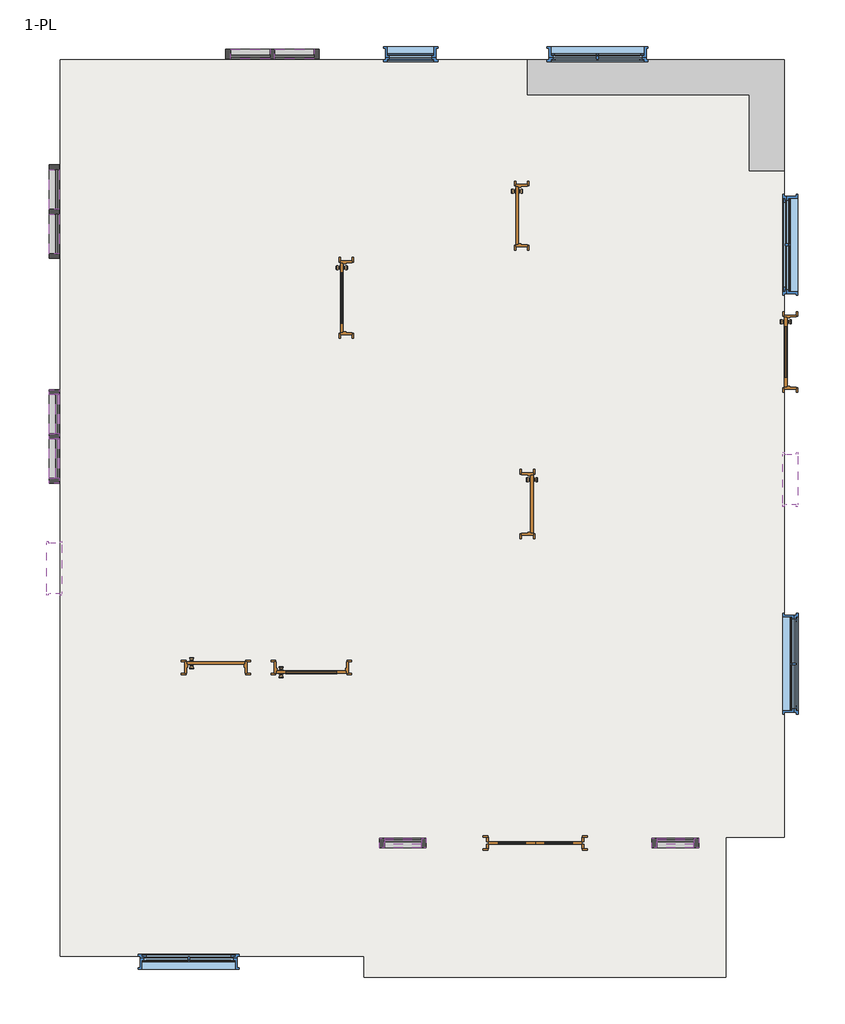
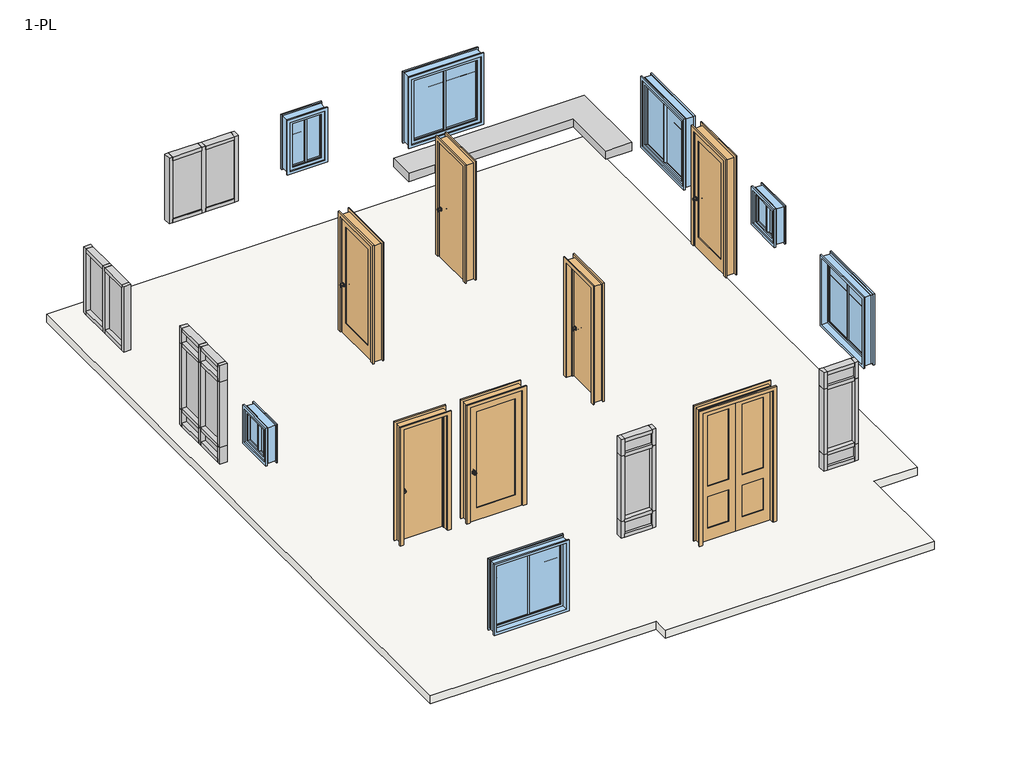
# One storey: 51 members, 16 plates, 7 doors, 7 windows, 1 furniture element, 1 slab.
"""IFC4 building model written with IfcOpenShell, lengths in millimetres."""

from ifc_helpers import new_model, si_unit, frame, origin, place, context, project, spatial, polyline, outline, extrude, transform, mapped, element, save
from components import door_interior_double_pocket_2_panel_wood_4_x8_0aea24c3, door_interior_single_1_panel_wood_3_x7_5a860750, door_2b62d641, door_6764305a, casework_1_casework_1_03657681, member_86d06fe4, member_323df77c, member_3c3dc66a, member_75074519, member_0b7646a3, member_75d1e245, member_aaa03826, member_2b49869a, system_panel_glazed_cd2dd794, system_panel_glazed_63160b6e, system_panel_glazed_17912afe, system_panel_glazed_1715a493, system_panel_solid_a8a40995, yu_window_casement_1219x1219_b0d26e5b, yu_window_casement_610x610_b7484dfd, yu_window_casement_610x914_cab7b646

model = new_model("IFC4")

# Units and contexts
model_context = context("Model", 3, world=origin())
ifc_project = project(units=[si_unit("LENGTHUNIT", "METRE", prefix="MILLI")], contexts=[model_context])

# Site, building, storey
site = spatial("IfcSite", under=ifc_project)
building = spatial("IfcBuilding", under=site)
storey = spatial("IfcBuildingStorey", under=building, Name="1-PL", Elevation=609.6)

# Doors
placement = place(None, origin())
door_interior_double_pocket_2_panel_wood_4_x8_shape = door_interior_double_pocket_2_panel_wood_4_x8_0aea24c3(model_context)
element("IfcDoor", 1, ObjectType="Door-Interior-Double-Pocket-2_Panel-Wood : 4'x8'", at=placement, inside=storey, context=model_context, shape_type="MappedRepresentation", body=[
    mapped(door_interior_double_pocket_2_panel_wood_4_x8_shape, transform((456.1465688, 1034.5352197, 609.6), x_axis=(-1.0, 0.0, 0.0), y_axis=(0.0, -1.0, 0.0), z_axis=(0.0, 0.0, 1.0))),
])
door_interior_single_1_panel_wood_3_x7_shape = door_interior_single_1_panel_wood_3_x7_5a860750(model_context)
element("IfcDoor", 2, ObjectType="Door-Interior-Single-1_Panel-Wood : 3'x7'", at=placement, inside=storey, context=model_context, shape_type="MappedRepresentation", body=[
    mapped(door_interior_single_1_panel_wood_3_x7_shape, transform((-2464.8534312, 3317.3602197, 609.6), x_axis=(1.0, 0.0, 0.0), y_axis=(0.0, 1.0, 0.0), z_axis=(0.0, 0.0, 1.0))),
])
element("IfcDoor", 3, ObjectType="Door-Interior-Single-1_Panel-Wood : 3'x7'", at=placement, inside=storey, context=model_context, shape_type="MappedRepresentation", body=[
    mapped(door_interior_single_1_panel_wood_3_x7_shape, transform((-2010.8284312, 8140.986397, 609.6), x_axis=(0.0, -1.0, 0.0), y_axis=(1.0, 0.0, 0.0), z_axis=(0.0, 0.0, 1.0))),
])
element("IfcDoor", 4, ObjectType="Door-Interior-Single-1_Panel-Wood : 3'x7'", at=placement, inside=storey, context=model_context, shape_type="MappedRepresentation", body=[
    mapped(door_interior_single_1_panel_wood_3_x7_shape, transform((3780.3715688, 7435.3352197, 609.6), x_axis=(0.0, -1.0, 0.0), y_axis=(1.0, 0.0, 0.0), z_axis=(0.0, 0.0, 1.0))),
])
door_shape = door_2b62d641(model_context)
element("IfcDoor", 5, ObjectType="Door-Interior-Single-Flush_Panel-Wood : 2'6\" x 7'", at=placement, inside=storey, context=model_context, shape_type="MappedRepresentation", body=[
    mapped(door_shape, transform((-3709.4534312, 3323.7102197, 609.6), x_axis=(1.0, 0.0, 0.0), y_axis=(0.0, 1.0, 0.0), z_axis=(0.0, 0.0, 1.0))),
])
element("IfcDoor", 6, ObjectType="Door-Interior-Single-Flush_Panel-Wood : 2'6\" x 7'", at=placement, inside=storey, context=model_context, shape_type="MappedRepresentation", body=[
    mapped(door_shape, transform((357.7215688, 5454.1352197, 609.6), x_axis=(0.0, -1.0, 0.0), y_axis=(1.0, 0.0, 0.0), z_axis=(0.0, 0.0, 1.0))),
])
door_2_shape = door_6764305a(model_context)
element("IfcDoor", 7, ObjectType="Door-Interior-Single-Flush_Panel-Wood : 2'6\" x 7'", at=placement, inside=storey, context=model_context, shape_type="MappedRepresentation", body=[
    mapped(door_2_shape, transform((275.1715688, 9213.3352197, 609.6), x_axis=(0.0, -1.0, 0.0), y_axis=(1.0, 0.0, 0.0), z_axis=(0.0, 0.0, 1.0))),
])

# Furniture
casework_1_casework_1_shape = casework_1_casework_1_03657681(model_context)
element("IfcFurniture", 8, ObjectType="Casework 1 : Casework 1", at=placement, inside=storey, context=model_context, shape_type="MappedRepresentation", body=[
    mapped(casework_1_casework_1_shape, transform((0.0, 0.0, 0.0), x_axis=(1.0, 0.0, 0.0), y_axis=(0.0, 1.0, 0.0), z_axis=(0.0, 0.0, 1.0))),
])

# Members
member_shape = member_86d06fe4(model_context)
element("IfcMember", 9, ObjectType="Rectangular Mullion : 2.5\" x 5\" rectangular", at=placement, inside=storey, context=model_context, shape_type="MappedRepresentation", body=[
    mapped(member_shape, transform((-1029.7534312, 1034.5352197, 3048.0), x_axis=(0.0, 0.0, 1.0), y_axis=(0.0, -1.0, 0.0), z_axis=(1.0, 0.0, 0.0))),
])
element("IfcMember", 10, ObjectType="Rectangular Mullion : 2.5\" x 5\" rectangular", at=placement, inside=storey, context=model_context, shape_type="MappedRepresentation", body=[
    mapped(member_shape, transform((2526.2465688, 1034.5352197, 3048.0), x_axis=(0.0, 0.0, 1.0), y_axis=(0.0, -1.0, 0.0), z_axis=(1.0, 0.0, 0.0))),
])
element("IfcMember", 11, ObjectType="Rectangular Mullion : 2.5\" x 5\" rectangular", at=placement, inside=storey, context=model_context, shape_type="MappedRepresentation", body=[
    mapped(member_shape, transform((-1512.3534312, 1034.5352197, 1219.2), x_axis=(0.0, 0.0, -1.0), y_axis=(0.0, -1.0, 0.0), z_axis=(-1.0, 0.0, 0.0))),
])
element("IfcMember", 12, ObjectType="Rectangular Mullion : 2.5\" x 5\" rectangular", at=placement, inside=storey, context=model_context, shape_type="MappedRepresentation", body=[
    mapped(member_shape, transform((2043.6465688, 1034.5352197, 1219.2), x_axis=(0.0, 0.0, -1.0), y_axis=(0.0, -1.0, 0.0), z_axis=(-1.0, 0.0, 0.0))),
])
member_2_shape = member_323df77c(model_context)
element("IfcMember", 13, ObjectType="Rectangular Mullion : 2.5\" x 5\" rectangular", at=placement, inside=storey, context=model_context, shape_type="MappedRepresentation", body=[
    mapped(member_2_shape, transform((-1029.7534312, 1034.5352197, 2743.2), x_axis=(0.0, 0.0, 1.0), y_axis=(0.0, -1.0, 0.0), z_axis=(1.0, 0.0, 0.0))),
])
element("IfcMember", 14, ObjectType="Rectangular Mullion : 2.5\" x 5\" rectangular", at=placement, inside=storey, context=model_context, shape_type="MappedRepresentation", body=[
    mapped(member_2_shape, transform((-1029.7534312, 1034.5352197, 1524.0), x_axis=(0.0, 0.0, 1.0), y_axis=(0.0, -1.0, 0.0), z_axis=(1.0, 0.0, 0.0))),
])
element("IfcMember", 15, ObjectType="Rectangular Mullion : 2.5\" x 5\" rectangular", at=placement, inside=storey, context=model_context, shape_type="MappedRepresentation", body=[
    mapped(member_2_shape, transform((2526.2465688, 1034.5352197, 2743.2), x_axis=(0.0, 0.0, 1.0), y_axis=(0.0, -1.0, 0.0), z_axis=(1.0, 0.0, 0.0))),
])
element("IfcMember", 16, ObjectType="Rectangular Mullion : 2.5\" x 5\" rectangular", at=placement, inside=storey, context=model_context, shape_type="MappedRepresentation", body=[
    mapped(member_2_shape, transform((2526.2465688, 1034.5352197, 1524.0), x_axis=(0.0, 0.0, 1.0), y_axis=(0.0, -1.0, 0.0), z_axis=(1.0, 0.0, 0.0))),
])
member_3_shape = member_3c3dc66a(model_context)
element("IfcMember", 17, ObjectType="Rectangular Mullion : 2.5\" x 5\" rectangular", at=placement, inside=storey, context=model_context, shape_type="MappedRepresentation", body=[
    mapped(member_3_shape, transform((-1575.8534312, 1034.5352197, 3048.0), x_axis=(-1.0, 0.0, 0.0), y_axis=(0.0, -1.0, 0.0), z_axis=(0.0, 0.0, 1.0))),
])
element("IfcMember", 18, ObjectType="Rectangular Mullion : 2.5\" x 5\" rectangular", at=placement, inside=storey, context=model_context, shape_type="MappedRepresentation", body=[
    mapped(member_3_shape, transform((1980.1465688, 1034.5352197, 3048.0), x_axis=(-1.0, 0.0, 0.0), y_axis=(0.0, -1.0, 0.0), z_axis=(0.0, 0.0, 1.0))),
])
element("IfcMember", 19, ObjectType="Rectangular Mullion : 2.5\" x 5\" rectangular", at=placement, inside=storey, context=model_context, shape_type="MappedRepresentation", body=[
    mapped(member_3_shape, transform((-5817.6534312, 6946.3852197, 3048.0), x_axis=(0.0, 1.0, 0.0), y_axis=(-1.0, 0.0, 0.0), z_axis=(0.0, 0.0, 1.0))),
])
element("IfcMember", 20, ObjectType="Rectangular Mullion : 2.5\" x 5\" rectangular", at=placement, inside=storey, context=model_context, shape_type="MappedRepresentation", body=[
    mapped(member_3_shape, transform((-966.2534312, 1034.5352197, 1219.2), x_axis=(1.0, 0.0, 0.0), y_axis=(0.0, -1.0, 0.0), z_axis=(0.0, 0.0, -1.0))),
])
element("IfcMember", 21, ObjectType="Rectangular Mullion : 2.5\" x 5\" rectangular", at=placement, inside=storey, context=model_context, shape_type="MappedRepresentation", body=[
    mapped(member_3_shape, transform((2589.7465688, 1034.5352197, 1219.2), x_axis=(1.0, 0.0, 0.0), y_axis=(0.0, -1.0, 0.0), z_axis=(0.0, 0.0, -1.0))),
])
element("IfcMember", 22, ObjectType="Rectangular Mullion : 2.5\" x 5\" rectangular", at=placement, inside=storey, context=model_context, shape_type="MappedRepresentation", body=[
    mapped(member_3_shape, transform((-5817.6534312, 5727.1852197, 1219.2), x_axis=(0.0, -1.0, 0.0), y_axis=(-1.0, 0.0, 0.0), z_axis=(0.0, 0.0, -1.0))),
])
element("IfcMember", 23, ObjectType="Rectangular Mullion : 2.5\" x 5\" rectangular", at=placement, inside=storey, context=model_context, shape_type="MappedRepresentation", body=[
    mapped(member_3_shape, transform((-966.2534312, 1034.5352197, 2743.2), x_axis=(1.0, 0.0, 0.0), y_axis=(0.0, -1.0, 0.0), z_axis=(0.0, 0.0, -1.0))),
])
element("IfcMember", 24, ObjectType="Rectangular Mullion : 2.5\" x 5\" rectangular", at=placement, inside=storey, context=model_context, shape_type="MappedRepresentation", body=[
    mapped(member_3_shape, transform((2589.7465688, 1034.5352197, 2743.2), x_axis=(1.0, 0.0, 0.0), y_axis=(0.0, -1.0, 0.0), z_axis=(0.0, 0.0, -1.0))),
])
element("IfcMember", 25, ObjectType="Rectangular Mullion : 2.5\" x 5\" rectangular", at=placement, inside=storey, context=model_context, shape_type="MappedRepresentation", body=[
    mapped(member_3_shape, transform((-5817.6534312, 5727.1852197, 2743.2), x_axis=(0.0, -1.0, 0.0), y_axis=(-1.0, 0.0, 0.0), z_axis=(0.0, 0.0, -1.0))),
])
member_4_shape = member_75074519(model_context)
element("IfcMember", 26, ObjectType="Rectangular Mullion : 2.5\" x 5\" rectangular", at=placement, inside=storey, context=model_context, shape_type="MappedRepresentation", body=[
    mapped(member_4_shape, transform((-966.2534312, 1034.5352197, 1524.0), x_axis=(1.0, 0.0, 0.0), y_axis=(0.0, -1.0, 0.0), z_axis=(0.0, 0.0, -1.0))),
])
element("IfcMember", 27, ObjectType="Rectangular Mullion : 2.5\" x 5\" rectangular", at=placement, inside=storey, context=model_context, shape_type="MappedRepresentation", body=[
    mapped(member_4_shape, transform((2589.7465688, 1034.5352197, 1524.0), x_axis=(1.0, 0.0, 0.0), y_axis=(0.0, -1.0, 0.0), z_axis=(0.0, 0.0, -1.0))),
])
element("IfcMember", 28, ObjectType="Rectangular Mullion : 2.5\" x 5\" rectangular", at=placement, inside=storey, context=model_context, shape_type="MappedRepresentation", body=[
    mapped(member_4_shape, transform((-5817.6534312, 5727.1852197, 1524.0), x_axis=(0.0, -1.0, 0.0), y_axis=(-1.0, 0.0, 0.0), z_axis=(0.0, 0.0, -1.0))),
])
element("IfcMember", 29, ObjectType="Rectangular Mullion : 2.5\" x 5\" rectangular", at=placement, inside=storey, context=model_context, shape_type="MappedRepresentation", body=[
    mapped(member_4_shape, transform((-1575.8534312, 1034.5352197, 2743.2), x_axis=(-1.0, 0.0, 0.0), y_axis=(0.0, -1.0, 0.0), z_axis=(0.0, 0.0, 1.0))),
])
element("IfcMember", 30, ObjectType="Rectangular Mullion : 2.5\" x 5\" rectangular", at=placement, inside=storey, context=model_context, shape_type="MappedRepresentation", body=[
    mapped(member_4_shape, transform((1980.1465688, 1034.5352197, 2743.2), x_axis=(-1.0, 0.0, 0.0), y_axis=(0.0, -1.0, 0.0), z_axis=(0.0, 0.0, 1.0))),
])
element("IfcMember", 31, ObjectType="Rectangular Mullion : 2.5\" x 5\" rectangular", at=placement, inside=storey, context=model_context, shape_type="MappedRepresentation", body=[
    mapped(member_4_shape, transform((-5817.6534312, 6946.3852197, 2743.2), x_axis=(0.0, 1.0, 0.0), y_axis=(-1.0, 0.0, 0.0), z_axis=(0.0, 0.0, 1.0))),
])
element("IfcMember", 32, ObjectType="Rectangular Mullion : 2.5\" x 5\" rectangular", at=placement, inside=storey, context=model_context, shape_type="MappedRepresentation", body=[
    mapped(member_3_shape, transform((-1575.8534312, 1034.5352197, 1524.0), x_axis=(-1.0, 0.0, 0.0), y_axis=(0.0, -1.0, 0.0), z_axis=(0.0, 0.0, 1.0))),
])
element("IfcMember", 33, ObjectType="Rectangular Mullion : 2.5\" x 5\" rectangular", at=placement, inside=storey, context=model_context, shape_type="MappedRepresentation", body=[
    mapped(member_3_shape, transform((1980.1465688, 1034.5352197, 1524.0), x_axis=(-1.0, 0.0, 0.0), y_axis=(0.0, -1.0, 0.0), z_axis=(0.0, 0.0, 1.0))),
])
element("IfcMember", 34, ObjectType="Rectangular Mullion : 2.5\" x 5\" rectangular", at=placement, inside=storey, context=model_context, shape_type="MappedRepresentation", body=[
    mapped(member_3_shape, transform((-5817.6534312, 6946.3852197, 1524.0), x_axis=(0.0, 1.0, 0.0), y_axis=(-1.0, 0.0, 0.0), z_axis=(0.0, 0.0, 1.0))),
])
member_5_shape = member_0b7646a3(model_context)
element("IfcMember", 35, ObjectType="Rectangular Mullion : 2.5\" x 5\" rectangular", at=placement, inside=storey, context=model_context, shape_type="MappedRepresentation", body=[
    mapped(member_5_shape, transform((-5817.6534312, 5790.6852197, 3048.0), x_axis=(0.0, 0.0, 1.0), y_axis=(-1.0, 0.0, 0.0), z_axis=(0.0, -1.0, 0.0))),
])
element("IfcMember", 36, ObjectType="Rectangular Mullion : 2.5\" x 5\" rectangular", at=placement, inside=storey, context=model_context, shape_type="MappedRepresentation", body=[
    mapped(member_5_shape, transform((-5817.6534312, 6368.5352197, 3048.0), x_axis=(0.0, 0.0, 1.0), y_axis=(-1.0, 0.0, 0.0), z_axis=(0.0, -1.0, 0.0))),
])
element("IfcMember", 37, ObjectType="Rectangular Mullion : 2.5\" x 5\" rectangular", at=placement, inside=storey, context=model_context, shape_type="MappedRepresentation", body=[
    mapped(member_5_shape, transform((-5817.6534312, 8718.0352197, 2743.2), x_axis=(0.0, 0.0, 1.0), y_axis=(-1.0, 0.0, 0.0), z_axis=(0.0, -1.0, 0.0))),
])
element("IfcMember", 38, ObjectType="Rectangular Mullion : 2.5\" x 5\" rectangular", at=placement, inside=storey, context=model_context, shape_type="MappedRepresentation", body=[
    mapped(member_5_shape, transform((-5817.6534312, 9295.8852197, 2743.2), x_axis=(0.0, 0.0, 1.0), y_axis=(-1.0, 0.0, 0.0), z_axis=(0.0, -1.0, 0.0))),
])
element("IfcMember", 39, ObjectType="Rectangular Mullion : 2.5\" x 5\" rectangular", at=placement, inside=storey, context=model_context, shape_type="MappedRepresentation", body=[
    mapped(member_5_shape, transform((-3518.9534312, 11321.5352197, 2743.2), x_axis=(0.0, 0.0, 1.0), y_axis=(0.0, 1.0, 0.0), z_axis=(-1.0, 0.0, 0.0))),
])
element("IfcMember", 40, ObjectType="Rectangular Mullion : 2.5\" x 5\" rectangular", at=placement, inside=storey, context=model_context, shape_type="MappedRepresentation", body=[
    mapped(member_5_shape, transform((-2941.1034312, 11321.5352197, 2743.2), x_axis=(0.0, 0.0, 1.0), y_axis=(0.0, 1.0, 0.0), z_axis=(-1.0, 0.0, 0.0))),
])
element("IfcMember", 41, ObjectType="Rectangular Mullion : 2.5\" x 5\" rectangular", at=placement, inside=storey, context=model_context, shape_type="MappedRepresentation", body=[
    mapped(member_5_shape, transform((-5817.6534312, 6882.8852197, 1219.2), x_axis=(0.0, 0.0, -1.0), y_axis=(-1.0, 0.0, 0.0), z_axis=(0.0, 1.0, 0.0))),
])
element("IfcMember", 42, ObjectType="Rectangular Mullion : 2.5\" x 5\" rectangular", at=placement, inside=storey, context=model_context, shape_type="MappedRepresentation", body=[
    mapped(member_5_shape, transform((-5817.6534312, 6305.0352197, 1219.2), x_axis=(0.0, 0.0, -1.0), y_axis=(-1.0, 0.0, 0.0), z_axis=(0.0, 1.0, 0.0))),
])
element("IfcMember", 43, ObjectType="Rectangular Mullion : 2.5\" x 5\" rectangular", at=placement, inside=storey, context=model_context, shape_type="MappedRepresentation", body=[
    mapped(member_5_shape, transform((-5817.6534312, 9810.2352197, 1524.0), x_axis=(0.0, 0.0, -1.0), y_axis=(-1.0, 0.0, 0.0), z_axis=(0.0, 1.0, 0.0))),
])
element("IfcMember", 44, ObjectType="Rectangular Mullion : 2.5\" x 5\" rectangular", at=placement, inside=storey, context=model_context, shape_type="MappedRepresentation", body=[
    mapped(member_5_shape, transform((-5817.6534312, 9232.3852197, 1524.0), x_axis=(0.0, 0.0, -1.0), y_axis=(-1.0, 0.0, 0.0), z_axis=(0.0, 1.0, 0.0))),
])
element("IfcMember", 45, ObjectType="Rectangular Mullion : 2.5\" x 5\" rectangular", at=placement, inside=storey, context=model_context, shape_type="MappedRepresentation", body=[
    mapped(member_5_shape, transform((-2426.7534312, 11321.5352197, 1524.0), x_axis=(0.0, 0.0, -1.0), y_axis=(0.0, 1.0, 0.0), z_axis=(1.0, 0.0, 0.0))),
])
element("IfcMember", 46, ObjectType="Rectangular Mullion : 2.5\" x 5\" rectangular", at=placement, inside=storey, context=model_context, shape_type="MappedRepresentation", body=[
    mapped(member_5_shape, transform((-3004.6034312, 11321.5352197, 1524.0), x_axis=(0.0, 0.0, -1.0), y_axis=(0.0, 1.0, 0.0), z_axis=(1.0, 0.0, 0.0))),
])
member_6_shape = member_75d1e245(model_context)
element("IfcMember", 47, ObjectType="Rectangular Mullion : 2.5\" x 5\" rectangular", at=placement, inside=storey, context=model_context, shape_type="MappedRepresentation", body=[
    mapped(member_6_shape, transform((-5817.6534312, 6336.7852197, 1219.2), x_axis=(0.0, -1.0, 0.0), y_axis=(-1.0, 0.0, 0.0), z_axis=(0.0, 0.0, -1.0))),
])
member_7_shape = member_aaa03826(model_context)
element("IfcMember", 48, ObjectType="Rectangular Mullion : 2.5\" x 5\" rectangular", at=placement, inside=storey, context=model_context, shape_type="MappedRepresentation", body=[
    mapped(member_7_shape, transform((-5817.6534312, 6368.5352197, 2743.2), x_axis=(0.0, 0.0, 1.0), y_axis=(-1.0, 0.0, 0.0), z_axis=(0.0, -1.0, 0.0))),
])
element("IfcMember", 49, ObjectType="Rectangular Mullion : 2.5\" x 5\" rectangular", at=placement, inside=storey, context=model_context, shape_type="MappedRepresentation", body=[
    mapped(member_7_shape, transform((-5817.6534312, 5790.6852197, 2743.2), x_axis=(0.0, 0.0, 1.0), y_axis=(-1.0, 0.0, 0.0), z_axis=(0.0, -1.0, 0.0))),
])
element("IfcMember", 50, ObjectType="Rectangular Mullion : 2.5\" x 5\" rectangular", at=placement, inside=storey, context=model_context, shape_type="MappedRepresentation", body=[
    mapped(member_7_shape, transform((-5817.6534312, 6368.5352197, 1524.0), x_axis=(0.0, 0.0, 1.0), y_axis=(-1.0, 0.0, 0.0), z_axis=(0.0, -1.0, 0.0))),
])
element("IfcMember", 51, ObjectType="Rectangular Mullion : 2.5\" x 5\" rectangular", at=placement, inside=storey, context=model_context, shape_type="MappedRepresentation", body=[
    mapped(member_7_shape, transform((-5817.6534312, 5790.6852197, 1524.0), x_axis=(0.0, 0.0, 1.0), y_axis=(-1.0, 0.0, 0.0), z_axis=(0.0, -1.0, 0.0))),
])
element("IfcMember", 52, ObjectType="Rectangular Mullion : 2.5\" x 5\" rectangular", at=placement, inside=storey, context=model_context, shape_type="MappedRepresentation", body=[
    mapped(member_6_shape, transform((-5817.6534312, 6336.7852197, 2743.2), x_axis=(0.0, -1.0, 0.0), y_axis=(-1.0, 0.0, 0.0), z_axis=(0.0, 0.0, -1.0))),
])
member_8_shape = member_2b49869a(model_context)
element("IfcMember", 53, ObjectType="Rectangular Mullion : 2.5\" x 5\" rectangular", at=placement, inside=storey, context=model_context, shape_type="MappedRepresentation", body=[
    mapped(member_8_shape, transform((-5817.6534312, 6336.7852197, 1524.0), x_axis=(0.0, -1.0, 0.0), y_axis=(-1.0, 0.0, 0.0), z_axis=(0.0, 0.0, -1.0))),
])
element("IfcMember", 54, ObjectType="Rectangular Mullion : 2.5\" x 5\" rectangular", at=placement, inside=storey, context=model_context, shape_type="MappedRepresentation", body=[
    mapped(member_8_shape, transform((-5817.6534312, 9264.1352197, 1524.0), x_axis=(0.0, -1.0, 0.0), y_axis=(-1.0, 0.0, 0.0), z_axis=(0.0, 0.0, -1.0))),
])
element("IfcMember", 55, ObjectType="Rectangular Mullion : 2.5\" x 5\" rectangular", at=placement, inside=storey, context=model_context, shape_type="MappedRepresentation", body=[
    mapped(member_8_shape, transform((-2972.8534312, 11321.5352197, 1524.0), x_axis=(-1.0, 0.0, 0.0), y_axis=(0.0, 1.0, 0.0), z_axis=(0.0, 0.0, -1.0))),
])
element("IfcMember", 56, ObjectType="Rectangular Mullion : 2.5\" x 5\" rectangular", at=placement, inside=storey, context=model_context, shape_type="MappedRepresentation", body=[
    mapped(member_4_shape, transform((-5817.6534312, 9873.7352197, 2743.2), x_axis=(0.0, 1.0, 0.0), y_axis=(-1.0, 0.0, 0.0), z_axis=(0.0, 0.0, 1.0))),
])
element("IfcMember", 57, ObjectType="Rectangular Mullion : 2.5\" x 5\" rectangular", at=placement, inside=storey, context=model_context, shape_type="MappedRepresentation", body=[
    mapped(member_4_shape, transform((-2363.2534312, 11321.5352197, 2743.2), x_axis=(1.0, 0.0, 0.0), y_axis=(0.0, 1.0, 0.0), z_axis=(0.0, 0.0, 1.0))),
])
element("IfcMember", 58, ObjectType="Rectangular Mullion : 2.5\" x 5\" rectangular", at=placement, inside=storey, context=model_context, shape_type="MappedRepresentation", body=[
    mapped(member_4_shape, transform((-5817.6534312, 8654.5352197, 1524.0), x_axis=(0.0, -1.0, 0.0), y_axis=(-1.0, 0.0, 0.0), z_axis=(0.0, 0.0, -1.0))),
])
element("IfcMember", 59, ObjectType="Rectangular Mullion : 2.5\" x 5\" rectangular", at=placement, inside=storey, context=model_context, shape_type="MappedRepresentation", body=[
    mapped(member_4_shape, transform((-3582.4534312, 11321.5352197, 1524.0), x_axis=(-1.0, 0.0, 0.0), y_axis=(0.0, 1.0, 0.0), z_axis=(0.0, 0.0, -1.0))),
])

# Plates
system_panel_glazed_shape = system_panel_glazed_cd2dd794(model_context)
element("IfcPlate", 60, ObjectType="System Panel : Glazed", at=placement, inside=storey, context=model_context, shape_type="MappedRepresentation", body=[
    mapped(system_panel_glazed_shape, transform((-1271.0534312, 1034.5352197, 1555.75), x_axis=(1.0, 0.0, 0.0), y_axis=(0.0, 1.0, 0.0), z_axis=(0.0, 0.0, 1.0))),
])
element("IfcPlate", 61, ObjectType="System Panel : Glazed", at=placement, inside=storey, context=model_context, shape_type="MappedRepresentation", body=[
    mapped(system_panel_glazed_shape, transform((2284.9465688, 1034.5352197, 1555.75), x_axis=(1.0, 0.0, 0.0), y_axis=(0.0, 1.0, 0.0), z_axis=(0.0, 0.0, 1.0))),
])
system_panel_glazed_2_shape = system_panel_glazed_63160b6e(model_context)
element("IfcPlate", 62, ObjectType="System Panel : Glazed", at=placement, inside=storey, context=model_context, shape_type="MappedRepresentation", body=[
    mapped(system_panel_glazed_2_shape, transform((-5817.6534312, 6625.7102197, 1282.7), x_axis=(0.0, -1.0, 0.0), y_axis=(1.0, 0.0, 0.0), z_axis=(0.0, 0.0, 1.0))),
])
element("IfcPlate", 63, ObjectType="System Panel : Glazed", at=placement, inside=storey, context=model_context, shape_type="MappedRepresentation", body=[
    mapped(system_panel_glazed_2_shape, transform((-5817.6534312, 6047.8602197, 1282.7), x_axis=(0.0, -1.0, 0.0), y_axis=(1.0, 0.0, 0.0), z_axis=(0.0, 0.0, 1.0))),
])
element("IfcPlate", 64, ObjectType="System Panel : Glazed", at=placement, inside=storey, context=model_context, shape_type="MappedRepresentation", body=[
    mapped(system_panel_glazed_2_shape, transform((-5817.6534312, 6625.7102197, 2774.95), x_axis=(0.0, -1.0, 0.0), y_axis=(1.0, 0.0, 0.0), z_axis=(0.0, 0.0, 1.0))),
])
element("IfcPlate", 65, ObjectType="System Panel : Glazed", at=placement, inside=storey, context=model_context, shape_type="MappedRepresentation", body=[
    mapped(system_panel_glazed_2_shape, transform((-5817.6534312, 6047.8602197, 2774.95), x_axis=(0.0, -1.0, 0.0), y_axis=(1.0, 0.0, 0.0), z_axis=(0.0, 0.0, 1.0))),
])
system_panel_glazed_3_shape = system_panel_glazed_17912afe(model_context)
element("IfcPlate", 66, ObjectType="System Panel : Glazed", at=placement, inside=storey, context=model_context, shape_type="MappedRepresentation", body=[
    mapped(system_panel_glazed_3_shape, transform((-5817.6534312, 6625.7102197, 1555.75), x_axis=(0.0, -1.0, 0.0), y_axis=(1.0, 0.0, 0.0), z_axis=(0.0, 0.0, 1.0))),
])
element("IfcPlate", 67, ObjectType="System Panel : Glazed", at=placement, inside=storey, context=model_context, shape_type="MappedRepresentation", body=[
    mapped(system_panel_glazed_3_shape, transform((-5817.6534312, 6047.8602197, 1555.75), x_axis=(0.0, -1.0, 0.0), y_axis=(1.0, 0.0, 0.0), z_axis=(0.0, 0.0, 1.0))),
])
system_panel_glazed_4_shape = system_panel_glazed_1715a493(model_context)
element("IfcPlate", 68, ObjectType="System Panel : Glazed", at=placement, inside=storey, context=model_context, shape_type="MappedRepresentation", body=[
    mapped(system_panel_glazed_4_shape, transform((-5817.6534312, 9553.0602197, 1587.5), x_axis=(0.0, -1.0, 0.0), y_axis=(1.0, 0.0, 0.0), z_axis=(0.0, 0.0, 1.0))),
])
element("IfcPlate", 69, ObjectType="System Panel : Glazed", at=placement, inside=storey, context=model_context, shape_type="MappedRepresentation", body=[
    mapped(system_panel_glazed_4_shape, transform((-2683.9284312, 11321.5352197, 1587.5), x_axis=(-1.0, 0.0, 0.0), y_axis=(0.0, -1.0, 0.0), z_axis=(0.0, 0.0, 1.0))),
])
element("IfcPlate", 70, ObjectType="System Panel : Glazed", at=placement, inside=storey, context=model_context, shape_type="MappedRepresentation", body=[
    mapped(system_panel_glazed_4_shape, transform((-5817.6534312, 8975.2102197, 1587.5), x_axis=(0.0, -1.0, 0.0), y_axis=(1.0, 0.0, 0.0), z_axis=(0.0, 0.0, 1.0))),
])
element("IfcPlate", 71, ObjectType="System Panel : Glazed", at=placement, inside=storey, context=model_context, shape_type="MappedRepresentation", body=[
    mapped(system_panel_glazed_4_shape, transform((-3261.7784312, 11321.5352197, 1587.5), x_axis=(-1.0, 0.0, 0.0), y_axis=(0.0, -1.0, 0.0), z_axis=(0.0, 0.0, 1.0))),
])
system_panel_solid_shape = system_panel_solid_a8a40995(model_context)
element("IfcPlate", 72, ObjectType="System Panel : Solid", at=placement, inside=storey, context=model_context, shape_type="MappedRepresentation", body=[
    mapped(system_panel_solid_shape, transform((-1271.0534312, 1034.5352197, 1282.7), x_axis=(1.0, 0.0, 0.0), y_axis=(0.0, 1.0, 0.0), z_axis=(0.0, 0.0, 1.0))),
])
element("IfcPlate", 73, ObjectType="System Panel : Solid", at=placement, inside=storey, context=model_context, shape_type="MappedRepresentation", body=[
    mapped(system_panel_solid_shape, transform((2284.9465688, 1034.5352197, 1282.7), x_axis=(1.0, 0.0, 0.0), y_axis=(0.0, 1.0, 0.0), z_axis=(0.0, 0.0, 1.0))),
])
element("IfcPlate", 74, ObjectType="System Panel : Solid", at=placement, inside=storey, context=model_context, shape_type="MappedRepresentation", body=[
    mapped(system_panel_solid_shape, transform((-1271.0534312, 1034.5352197, 2774.95), x_axis=(1.0, 0.0, 0.0), y_axis=(0.0, 1.0, 0.0), z_axis=(0.0, 0.0, 1.0))),
])
element("IfcPlate", 75, ObjectType="System Panel : Solid", at=placement, inside=storey, context=model_context, shape_type="MappedRepresentation", body=[
    mapped(system_panel_solid_shape, transform((2284.9465688, 1034.5352197, 2774.95), x_axis=(1.0, 0.0, 0.0), y_axis=(0.0, 1.0, 0.0), z_axis=(0.0, 0.0, 1.0))),
])

# Slab
element("IfcSlab", 76, ObjectType="6\" floor", at=placement, inside=storey, context=model_context, shape_type="SweptSolid", body=[
    extrude(outline(polyline([(3707.3465688, 11245.3352197), (3707.3465688, 1110.7352197), (2945.3465688, 1110.7352197), (2945.3465688, -718.0647803), (-1779.0534312, -718.0647803), (-1779.0534312, -438.6647803), (-5741.4534312, -438.6647803), (-5741.4534312, 11245.3352197), (3707.3465688, 11245.3352197)])), frame((0.0, 0.0, 457.2), z_axis=(0.0, 0.0, 1.0), x_axis=(1.0, 0.0, 0.0)), (0.0, 0.0, 1.0), 152.4),
])

# Windows
yu_window_casement_1219x1219_shape = yu_window_casement_1219x1219_b0d26e5b(model_context)
element("IfcWindow", 77, ObjectType="Yu_Window : Casement 1219x1219", at=placement, inside=storey, context=model_context, shape_type="MappedRepresentation", body=[
    mapped(yu_window_casement_1219x1219_shape, transform((1268.9465688, 11321.5352197, 924.0), x_axis=(-1.0, 0.0, 0.0), y_axis=(0.0, -1.0, 0.0), z_axis=(0.0, 0.0, 1.0))),
])
element("IfcWindow", 78, ObjectType="Yu_Window : Casement 1219x1219", at=placement, inside=storey, context=model_context, shape_type="MappedRepresentation", body=[
    mapped(yu_window_casement_1219x1219_shape, transform((3783.5465688, 8832.3352197, 924.0), x_axis=(0.0, 1.0, 0.0), y_axis=(-1.0, 0.0, 0.0), z_axis=(0.0, 0.0, 1.0))),
])
element("IfcWindow", 79, ObjectType="Yu_Window : Casement 1219x1219", at=placement, inside=storey, context=model_context, shape_type="MappedRepresentation", body=[
    mapped(yu_window_casement_1219x1219_shape, transform((3783.5465688, 3371.3352197, 924.0), x_axis=(0.0, -1.0, 0.0), y_axis=(1.0, 0.0, 0.0), z_axis=(0.0, 0.0, 1.0))),
])
element("IfcWindow", 80, ObjectType="Yu_Window : Casement 1219x1219", at=placement, inside=storey, context=model_context, shape_type="MappedRepresentation", body=[
    mapped(yu_window_casement_1219x1219_shape, transform((-4065.0534312, -514.8647803, 924.0), x_axis=(1.0, 0.0, 0.0), y_axis=(0.0, 1.0, 0.0), z_axis=(0.0, 0.0, 1.0))),
])
yu_window_casement_610x610_shape = yu_window_casement_610x610_b7484dfd(model_context)
element("IfcWindow", 81, ObjectType="Yu_Window : Casement 610x610", at=placement, inside=storey, context=model_context, shape_type="MappedRepresentation", body=[
    mapped(yu_window_casement_610x610_shape, transform((3783.5465688, 5771.6352197, 1533.6), x_axis=(0.0, 1.0, 0.0), y_axis=(-1.0, 0.0, 0.0), z_axis=(0.0, 0.0, 1.0))),
])
element("IfcWindow", 82, ObjectType="Yu_Window : Casement 610x610", at=placement, inside=storey, context=model_context, shape_type="MappedRepresentation", body=[
    mapped(yu_window_casement_610x610_shape, transform((-5817.6534312, 4615.9352197, 1533.6), x_axis=(0.0, 1.0, 0.0), y_axis=(-1.0, 0.0, 0.0), z_axis=(0.0, 0.0, 1.0))),
])
yu_window_casement_610x914_shape = yu_window_casement_610x914_cab7b646(model_context)
element("IfcWindow", 83, ObjectType="Yu_Window : Casement 610x914", at=placement, inside=storey, context=model_context, shape_type="MappedRepresentation", body=[
    mapped(yu_window_casement_610x914_shape, transform((-1169.4534312, 11321.5352197, 1178.8), x_axis=(-1.0, 0.0, 0.0), y_axis=(0.0, -1.0, 0.0), z_axis=(0.0, 0.0, 1.0))),
])

save(model, "model.ifc")

# Revit data of these elements
# Type "Door-Interior-Double-Pocket-2_Panel-Wood : 4'x8'"
#   Type Mark = "11"
#   Assembly Code = "C1020300"
#   Analytic Construction = "Wooden"
#   Top Rail = 0' - 4 11/16"
#   Thickness = 0' - 1 3/8"
#   Thermal Resistance (R) = 2.5876 (h·ft²·°F)/BTU
#   Stiles = 0' - 4 3/4"
#   Rough Width = 8' - 2"
#   Rough Height = 8' - 4 1/2"
#   Panel Width = 2' - 0"
#   Lock Rail = 0' - 7 1/2"
#   Location [instance default] = 2' - 1"
#   Height = 8' - 0"
#   Width = 4' - 0"
#   Heat Transfer Coefficient (U) = 0.3865 BTU/(h·ft²·°F)
#   Bottom Rail = 0' - 9 1/8"
#   Panel Open [instance default] = no
#   Trim Material = Cherry
#   Panel Material = Cherry
#   Frame Material = Cherry
#   Visual Light Transmittance = 0
#   Solar Heat Gain Coefficient = 0
#   Wall Closure = (empty or 0)
#   Function = (empty or 0)
# Type "Door-Interior-Single-1_Panel-Wood : 3'x7'"
#   Type Mark = "9"
#   Assembly Code = "C1020300"
#   Analytic Construction = "Wooden"
#   Top Rail = 0' - 4 11/16"
#   Thickness = 0' - 1 3/8"
#   Thermal Resistance (R) = 2.5876 (h·ft²·°F)/BTU
#   Swing Angle [instance default] = 90.00°
#   Stiles = 0' - 4 3/4"
#   Rough Width = 3' - 2"
#   Rough Height = 7' - 1"
#   Height = 7' - 0"
#   Width = 3' - 0"
#   Heat Transfer Coefficient (U) = 0.3865 BTU/(h·ft²·°F)
#   Bottom Rail = 0' - 9 1/8"
#   Trim Material = Cherry
#   Panel Material = Cherry
#   Frame Material = Cherry
#   Door Handle Material = Aluminum
#   Visual Light Transmittance = 0
#   Solar Heat Gain Coefficient = 0
#   Wall Closure = (empty or 0)
#   Function = (empty or 0)
# Type "Door-Interior-Single-Flush_Panel-Wood : 2'6\" x 7'"
#   Type Mark = "13"
#   Assembly Code = "C1020300"
#   Analytic Construction = "Wooden"
#   Thickness = 0' - 1 3/8"
#   Thermal Resistance (R) = 2.5876 (h·ft²·°F)/BTU
#   Swing Angle [instance default] = 90.00°
#   Rough Width = 2' - 8"
#   Rough Height = 7' - 1"
#   Height = 7' - 0"
#   Width = 2' - 6"
#   Heat Transfer Coefficient (U) = 0.3865 BTU/(h·ft²·°F)
#   Trim Material = Cherry
#   Panel Material = Cherry
#   Frame Material = Cherry
#   Door Handle Material = Aluminum
#   Visual Light Transmittance = 0
#   Solar Heat Gain Coefficient = 0
#   Wall Closure = (empty or 0)
#   Function = (empty or 0)
# Type "Rectangular Mullion : 2.5\" x 5\" rectangular"
#   built-in parameter 1007304 = 0.416667 (stored number, unit not read)
#   built-in parameter 1007301 = 0.104167 (stored number, unit not read)
#   built-in parameter 1007300 = 0.104167 (stored number, unit not read)
# Type "System Panel : Glazed"
#   Construction Type Id = "GSP4R"
#   Analytic Construction = "1/8 in Pilkington single glazing"
#   Visual Light Transmittance = 0.9
#   Solar Heat Gain Coefficient = 0.86
#   Heat Transfer Coefficient (U) = 1.18115 BTU/(h·ft²·°F)
#   Define Thermal Properties by = 1
# Type "System Panel : Solid"
#   Construction Type Id = "MDOOR"
#   Analytic Construction = "Metal"
#   Visual Light Transmittance = 0
#   Solar Heat Gain Coefficient = 0
#   Heat Transfer Coefficient (U) = 0.651978 BTU/(h·ft²·°F)
#   Define Thermal Properties by = 1
# Type "6\" floor"
#   Assembly Code = "B1010"
#   Function = 0
#   Layers, outside or top first: 0' - 6" "00-9\" MAIN WALL" (function 1)
# Type "Yu_Window : Casement 1219x1219"
#   Type Mark = "22"
#   Analytic Construction = "<None>"
#   mullion 2 = 0' - 11.81102"
#   Window panel size 1 = 1' - 11.62205"
#   Offset = 0' - 0.98425"
#   Height = 4' - 0"
#   Default Sill Height = 1' - 11.62205"
#   Width = 4' - 0"
#   Define Thermal Properties by = 1
#   Interior material = none
#   Exterior material = none
#   Wall Closure = (empty or 0)
# Type "Yu_Window : Casement 610x610"
#   Type Mark = "25"
#   Analytic Construction = "<None>"
#   mullion 2 = 0' - 0"
#   Window panel size 1 = 0' - 8.85827"
#   Offset = 0' - 0.98425"
#   Height = 2' - 0"
#   Default Sill Height = 1' - 11.62205"
#   Width = 2' - 0"
#   Define Thermal Properties by = 1
#   Interior material = none
#   Exterior material = none
#   Wall Closure = (empty or 0)
# Type "Yu_Window : Casement 610x914"
#   Type Mark = "24"
#   Analytic Construction = "<None>"
#   mullion 2 = 0' - 11.81102"
#   Window panel size 1 = 0' - 11.81102"
#   Offset = 0' - 0.98425"
#   Height = 3' - 0"
#   Default Sill Height = 1' - 11.62205"
#   Width = 2' - 0"
#   Define Thermal Properties by = 1
#   Interior material = none
#   Exterior material = none
#   Wall Closure = (empty or 0)
# Element 1 (IfcDoor, "Door-Interior-Double-Pocket-2_Panel-Wood : 4'x8'")
#   Location = 2' - 1"
#   Panel Open = no
#   Phase Created = New Construction
#   Materials on its faces: "Cherry"
# Elements 2, 3, 4 (IfcDoor, "Door-Interior-Single-1_Panel-Wood : 3'x7'")
#   Swing Angle = 90.00°
#   Phase Created = New Construction
#   Materials on its faces: "Cherry", "Aluminum"
# Elements 5, 6, 7 (IfcDoor, "Door-Interior-Single-Flush_Panel-Wood : 2'6\" x 7'")
#   Swing Angle = 90.00°
#   Phase Created = New Construction
#   Materials on its faces: "Cherry", "Aluminum"
# Element 8 (IfcFurniture, "Casework 1 : Casework 1")
#   Phase Created = New Construction
# Elements 9, 10, 11, 12, 13, 14, 15, 16, 17, 18, 19, 20, 21, 22, 23, 24, 25, 26, 27, 28, 29, 30, 31, 32, 33, 34, 35, 36, 37, 38, 39, 40, 41, 42, 43, 44, 45, 46, 47, 48, 49, 50, 51, 52, 53, 54, 55, 56, 57, 58, 59 (IfcMember, "Rectangular Mullion : 2.5\" x 5\" rectangular")
#   Phase Created = New Construction
#   Materials on its faces: "Aluminum"
# Elements 60, 61, 62, 63, 64, 65, 66, 67, 68, 69, 70, 71 (IfcPlate, "System Panel : Glazed")
#   Phase Created = New Construction
#   Materials on its faces: "Glass"
# Elements 72, 73, 74, 75 (IfcPlate, "System Panel : Solid")
#   Phase Created = New Construction
#   Materials on its faces: "Default"
# Element 76 (IfcSlab, "6\" floor")
#   Height Offset From Level = 0' - 0"
#   Phase Created = New Construction
#   Materials on its faces: "00-9\" MAIN WALL"
# Element 77 (IfcWindow, "Yu_Window : Casement 1219x1219")
#   Mark = "7"
#   Phase Created = New Construction
#   Materials on its faces: "Glass"
# Element 78 (IfcWindow, "Yu_Window : Casement 1219x1219")
#   Mark = "8"
#   Phase Created = New Construction
#   Materials on its faces: "Glass"
# Element 79 (IfcWindow, "Yu_Window : Casement 1219x1219")
#   Mark = "9"
#   Phase Created = New Construction
#   Materials on its faces: "Glass"
# Element 80 (IfcWindow, "Yu_Window : Casement 1219x1219")
#   Mark = "10"
#   Phase Created = New Construction
#   Materials on its faces: "Glass"
# Element 81 (IfcWindow, "Yu_Window : Casement 610x610")
#   Mark = "4"
#   Phase Created = New Construction
#   Materials on its faces: "Glass"
# Element 82 (IfcWindow, "Yu_Window : Casement 610x610")
#   Mark = "5"
#   Phase Created = New Construction
#   Materials on its faces: "Glass"
# Element 83 (IfcWindow, "Yu_Window : Casement 610x914")
#   Mark = "6"
#   Phase Created = New Construction
#   Materials on its faces: "Glass"
# Materials
#   "Cherry": class "Wood", colour RGB 226 177 128, transparency 0, Description = "Prunus Serotina", Cost = 0
#   "Aluminum": class "Metal", colour RGB 247 247 247, transparency 0, Description = "Aluminum 6061", Cost = 0
#   "00-9\" MAIN WALL": class "Generic", colour RGB 244 244 244, transparency 0, Cost = 0
#   "Glass": class "Glass", colour RGB 0 128 192, transparency 0.75, Description = "Soda Lime Glass", Cost = 0
#   "Default": colour RGB 127 127 127, transparency 0, Cost = 0
